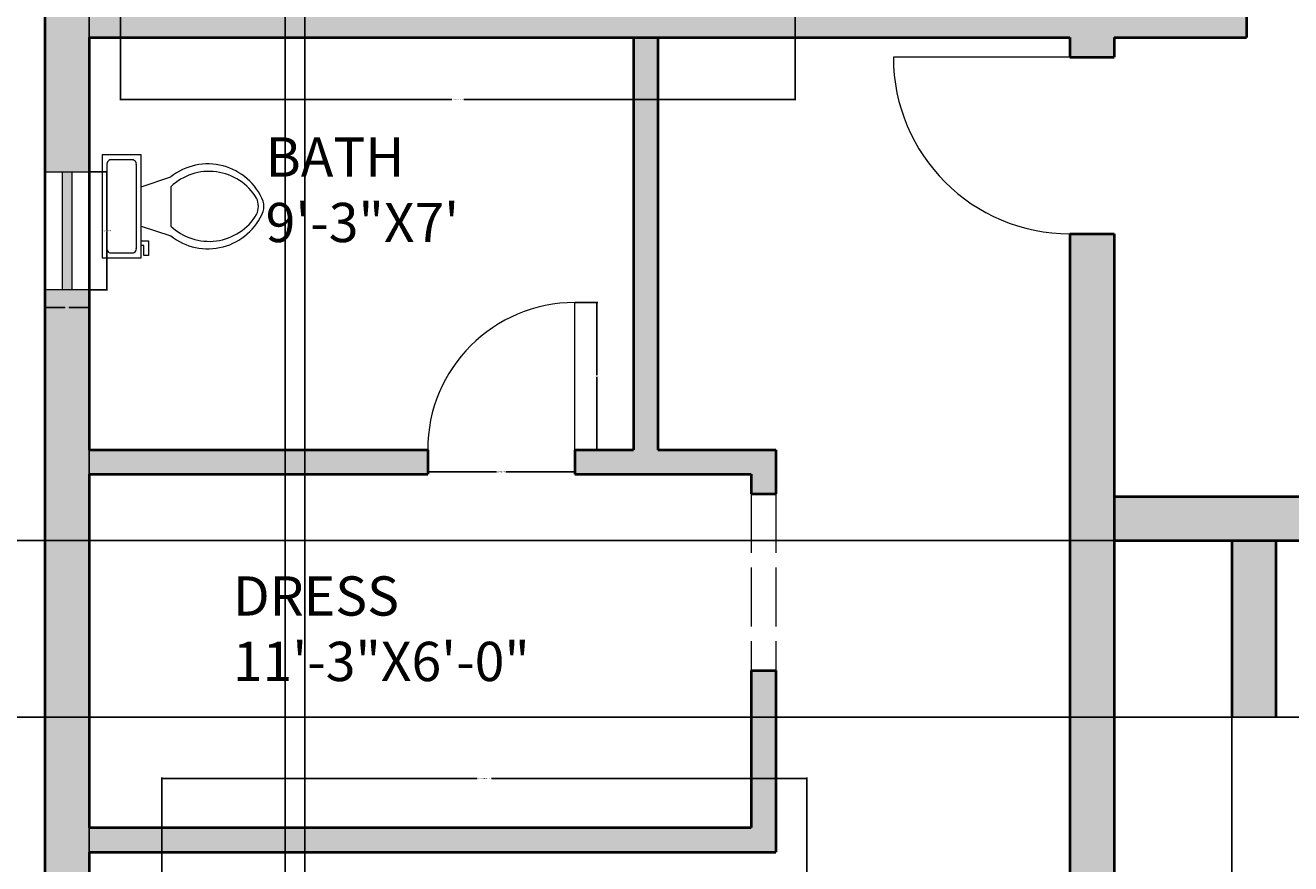
# Model space of a CAD drawing. Units: inches. Extents: x 2330 to 3943, y 1763 to 3461.
# Tile 9 of 40: x 2472 to 2730, y 2383 to 2554. Entities that reach past the tile are written whole.
import ezdxf

# ---------------------------------------------------------------- set-up
doc = ezdxf.new("R2010")
doc.units = ezdxf.units.IN
doc.linetypes.add('ACAD_ISO02W100', pattern=[15, 12, -3])
for name, color, linetype, lineweight in [('A-ANNO-DIMS', 2, 'Continuous', 18), ('A-AREA-IDEN', 7, 'Continuous', 18), ('A-DOOR', 4, 'Continuous', 18), ('A-FLOR', 7, 'Continuous', 25), ('A-FLOR-FIXT', 8, 'Continuous', 18), ('A-GLAZ', 4, 'Continuous', 18), ('A-WALL', 7, 'Continuous', 40), ('A-WALL-OVHD', 7, 'ACAD_ISO02W100', 18), ('A-WALL-PATT', 252, 'Continuous', 13)]:
    doc.layers.add(name, color=color, linetype=linetype, lineweight=lineweight)
doc.styles.get("Standard").update_dxf_attribs({"font": 'arial.ttf'})
doc.dimstyles.get("Standard").update_dxf_attribs({"dimtxt": 0.18, "dimasz": 0.18, "dimexe": 0.18, "dimexo": 0.0625, "dimgap": 0.09, "dimtad": 0, "dimtih": 1, "dimtoh": 1, "dimdec": 4, "dimzin": 0, "dimdsep": 46, "dimtxsty": 'Standard', "dimcen": 0.09, "dimadec": 0, "dimazin": 0, "dimtfac": 1, "dimtdec": 4, "dimtofl": 0, "dimtmove": 0, "dimatfit": 3, "dimfxl": 1, "dimtolj": 1, "dimtzin": 0, "dimarcsym": 0})

# ---------------------------------------------------------------- blocks, each defined once
blk = doc.blocks.new('*U9')
for p, q in [((9.5, -6), (9.5, -2)), ((-10, -8.5), (-8, -8.5)), ((-10, -9.5), (-10, -8.5)), ((-7, -9.5), (-10, -9.5)), ((-8, -8.5), (-8, -8)), ((-7, -8), (-7, -9.5)), ((-4, -8), (-6, -14)), ((4, -8), (6, -14)), ((4, -14), (-4, -14))]:
    blk.add_line(p, q)
blk.add_lwpolyline([(10.5, -8), (10.5, 0), (-10.5, 0), (-10.5, -8)], close=True)
for points in [[(-9.5, -2), (-9.5, -6)], [(8.5, -1), (-8.5, -1)], [(-8.5, -7), (8.5, -7)]]:
    blk.add_lwpolyline(points)
for centre, radius, start, end in [((-8.62, -1.88), 0.884, 81.8699, 188.1301), ((8.62, -1.88), 0.884, 351.8699, 98.1301), ((-8.62, -6.12), 0.884, 171.8699, 278.1301), ((8.62, -6.12), 0.884, 261.8699, 8.1301), ((3.52, -21.58), 12.17, 141.4691, 247.9714), ((4.2, -21.82), 11.33, 136.3677, 238.9468), ((-3.52, -21.58), 12.17, 292.0284, 38.5307), ((-4.2, -21.82), 11.33, 301.053, 43.6321), ((0, -27.88), 4, 245.7318, 294.2682), ((0, -29), 4, 254.8605, 285.1395)]:
    blk.add_arc(centre, radius, start, end)
blk = doc.blocks.new('DOOR-SINGLE-36IN')
blk.add_line((0, 0), (-36, 0))
blk.add_arc((0, 0), 36, 180, 270)
blk = doc.blocks.new('DOOR-SINGLE-30IN')
blk.add_line((0, 0), (0, 30))
blk.add_arc((0, 0), 30, 90, 180)
blk = doc.blocks.new('WINDOW-24IN')
h = blk.add_hatch(color=256)
h.dxf.hatch_style = 1
h.paths.add_polyline_path([(5.5, 24), (3.5, 24), (3.5, 0), (5.5, 0)])
for p, q in [((9, 24), (0, 24)), ((3.5, 24), (3.5, 0)), ((5.5, 24), (5.5, 0)), ((9, 0), (0, 0))]:
    blk.add_line(p, q)
blk = doc.blocks.new('*D31')
at = {"layer": 'A-ANNO-DIMS', "color": 0, "lineweight": -2, "transparency": 16777216}
for p, q in [((2553.7, 2467.09), (2553.7, 2462.47)), ((2583.7, 2467.09), (2583.7, 2462.47)), ((2553.88, 2462.65), (2567.77, 2462.65)), ((2583.52, 2462.65), (2569.64, 2462.65))]:
    blk.add_line(p, q, dxfattribs=at)
at = {"layer": 'A-ANNO-DIMS', "color": 0, "transparency": 16777216}
for points in [[(2553.88, 2462.68), (2553.88, 2462.62), (2553.7, 2462.65)], [(2583.52, 2462.68), (2583.52, 2462.62), (2583.7, 2462.65)]]:
    blk.add_solid(points, dxfattribs=at)
at = {"layer": 'Defpoints', "color": 0, "transparency": 16777216}
for p in [(2553.7, 2467.15), (2583.7, 2467.15), (2583.7, 2462.65)]:
    blk.add_point(p, dxfattribs=at)
at = {"layer": 'A-ANNO-DIMS', "color": 0, "transparency": 16777216, "insert": (2568.7, 2462.65), "char_height": 0.18, "attachment_point": 5}
blk.add_mtext('\\A1;DOOR 30 TYP.', dxfattribs=at)
blk = doc.blocks.new('*D32')
at = {"layer": 'A-ANNO-DIMS', "color": 0, "lineweight": -2, "transparency": 16777216}
for p, q in [((2583.77, 2497.15), (2588.38, 2497.15)), ((2588.2, 2496.97), (2588.2, 2482.33)), ((2588.2, 2467.33), (2588.2, 2481.97)), ((2583.77, 2467.15), (2588.38, 2467.15))]:
    blk.add_line(p, q, dxfattribs=at)
at = {"layer": 'A-ANNO-DIMS', "color": 0, "transparency": 16777216}
for points in [[(2588.17, 2496.97), (2588.23, 2496.97), (2588.2, 2497.15)], [(2588.17, 2467.33), (2588.23, 2467.33), (2588.2, 2467.15)]]:
    blk.add_solid(points, dxfattribs=at)
at = {"layer": 'Defpoints', "color": 0, "transparency": 16777216}
for p in [(2583.7, 2497.15), (2588.2, 2497.15), (2583.7, 2467.15)]:
    blk.add_point(p, dxfattribs=at)
at = {"layer": 'A-ANNO-DIMS', "color": 0, "transparency": 16777216, "insert": (2588.2, 2482.15), "char_height": 0.18, "attachment_point": 5}
blk.add_mtext('\\A1;30 TYP.', dxfattribs=at)
blk = doc.blocks.new('*D37')
at = {"layer": 'A-ANNO-DIMS', "color": 0, "lineweight": -2, "transparency": 16777216}
for p, q in [((2484.72, 2523.76), (2488.44, 2523.76)), ((2488.26, 2523.58), (2488.26, 2511.94)), ((2488.26, 2499.94), (2488.26, 2511.57)), ((2484.72, 2499.76), (2488.44, 2499.76))]:
    blk.add_line(p, q, dxfattribs=at)
at = {"layer": 'A-ANNO-DIMS', "color": 0, "transparency": 16777216}
for points in [[(2488.23, 2523.58), (2488.29, 2523.58), (2488.26, 2523.76)], [(2488.23, 2499.94), (2488.29, 2499.94), (2488.26, 2499.76)]]:
    blk.add_solid(points, dxfattribs=at)
at = {"layer": 'Defpoints', "color": 0, "transparency": 16777216}
for p in [(2484.66, 2523.76), (2488.26, 2523.76), (2484.66, 2499.76)]:
    blk.add_point(p, dxfattribs=at)
at = {"layer": 'A-ANNO-DIMS', "color": 0, "transparency": 16777216, "insert": (2488.26, 2511.76), "char_height": 0.18, "attachment_point": 5}
blk.add_mtext('\\A1;WINDOW 24 TYP.', dxfattribs=at)
blk = doc.blocks.new('*D38')
at = {"layer": 'A-ANNO-DIMS', "color": 0, "lineweight": -2, "transparency": 16777216}
for p, q in [((2475.66, 2499.69), (2475.66, 2495.98)), ((2484.66, 2499.69), (2484.66, 2495.98)), ((2475.84, 2496.16), (2479.7, 2496.16)), ((2484.48, 2496.16), (2480.62, 2496.16))]:
    blk.add_line(p, q, dxfattribs=at)
at = {"layer": 'A-ANNO-DIMS', "color": 0, "transparency": 16777216}
for points in [[(2475.84, 2496.19), (2475.84, 2496.13), (2475.66, 2496.16)], [(2484.48, 2496.19), (2484.48, 2496.13), (2484.66, 2496.16)]]:
    blk.add_solid(points, dxfattribs=at)
at = {"layer": 'Defpoints', "color": 0, "transparency": 16777216}
for p in [(2475.66, 2499.76), (2484.66, 2499.76), (2484.66, 2496.16)]:
    blk.add_point(p, dxfattribs=at)
at = {"layer": 'A-ANNO-DIMS', "color": 0, "transparency": 16777216, "insert": (2480.16, 2496.16), "char_height": 0.18, "attachment_point": 5}
blk.add_mtext('\\A1;9 TYP.', dxfattribs=at)
blk = doc.blocks.new('*D39')
at = {"layer": 'A-ANNO-DIMS', "color": 0, "lineweight": -2, "transparency": 16777216}
for p, q in [((2499.5, 2380.5), (2499.5, 2400.34)), ((2499.68, 2400.16), (2563.82, 2400.16)), ((2630.85, 2400.16), (2566.7, 2400.16)), ((2631.03, 2380.5), (2631.03, 2400.34))]:
    blk.add_line(p, q, dxfattribs=at)
at = {"layer": 'A-ANNO-DIMS', "color": 0, "transparency": 16777216}
for points in [[(2499.68, 2400.19), (2499.68, 2400.13), (2499.5, 2400.16)], [(2630.85, 2400.19), (2630.85, 2400.13), (2631.03, 2400.16)]]:
    blk.add_solid(points, dxfattribs=at)
at = {"layer": 'Defpoints', "color": 0, "transparency": 16777216}
for p in [(2631.03, 2400.16), (2499.5, 2380.43), (2631.03, 2380.43)]:
    blk.add_point(p, dxfattribs=at)
at = {"layer": 'A-ANNO-DIMS', "color": 0, "transparency": 16777216, "insert": (2565.26, 2400.16), "char_height": 0.18, "attachment_point": 5}
blk.add_mtext('\\A1;DOUBLE BED 132 TYP.', dxfattribs=at)
blk = doc.blocks.new('*D49')
at = {"layer": 'A-ANNO-DIMS', "color": 0, "lineweight": -2, "transparency": 16777216}
for p, q in [((2491.06, 2559.13), (2491.06, 2538.38)), ((2628.63, 2559.13), (2628.63, 2538.38)), ((2491.24, 2538.56), (2558.6, 2538.56)), ((2628.45, 2538.56), (2561.09, 2538.56))]:
    blk.add_line(p, q, dxfattribs=at)
at = {"layer": 'A-ANNO-DIMS', "color": 0, "transparency": 16777216}
for points in [[(2491.24, 2538.59), (2491.24, 2538.53), (2491.06, 2538.56)], [(2628.45, 2538.59), (2628.45, 2538.53), (2628.63, 2538.56)]]:
    blk.add_solid(points, dxfattribs=at)
at = {"layer": 'Defpoints', "color": 0, "transparency": 16777216}
for p in [(2491.06, 2559.19), (2628.63, 2559.19), (2491.06, 2538.56)]:
    blk.add_point(p, dxfattribs=at)
at = {"layer": 'A-ANNO-DIMS', "color": 0, "transparency": 16777216, "insert": (2559.84, 2538.56), "char_height": 0.18, "attachment_point": 5}
blk.add_mtext('\\A1;CORNER SOFA 138', dxfattribs=at)
blk = doc.blocks.new('*D62')
at = {"layer": 'A-ANNO-DIMS', "color": 0, "lineweight": -2, "transparency": 16777216}
for p, q in [((2475.6, 3162.65), (2330.5, 3162.65)), ((2330.68, 3162.47), (2330.68, 2687.58)), ((2330.68, 2212.33), (2330.68, 2687.22)), ((2475.6, 2212.15), (2330.5, 2212.15))]:
    blk.add_line(p, q, dxfattribs=at)
at = {"layer": 'A-ANNO-DIMS', "color": 0, "transparency": 16777216}
for points in [[(2330.65, 3162.47), (2330.71, 3162.47), (2330.68, 3162.65)], [(2330.65, 2212.33), (2330.71, 2212.33), (2330.68, 2212.15)]]:
    blk.add_solid(points, dxfattribs=at)
at = {"layer": 'Defpoints', "color": 0, "transparency": 16777216}
for p in [(2330.68, 3162.65), (2475.66, 3162.65), (2475.66, 2212.15)]:
    blk.add_point(p, dxfattribs=at)
at = {"layer": 'A-ANNO-DIMS', "color": 0, "transparency": 16777216, "insert": (2330.68, 2687.4), "char_height": 0.18, "attachment_point": 5}
blk.add_mtext('\\A1;950.5', dxfattribs=at)
blk = doc.blocks.new('*D77')
at = {"layer": 'A-ANNO-DIMS', "color": 0, "lineweight": -2, "transparency": 16777216}
for p, q in [((2717.66, 2412.59), (2717.66, 1901.2)), ((2944.66, 2412.59), (2944.66, 1901.2)), ((2717.84, 1901.38), (2830.87, 1901.38)), ((2944.48, 1901.38), (2831.45, 1901.38))]:
    blk.add_line(p, q, dxfattribs=at)
at = {"layer": 'A-ANNO-DIMS', "color": 0, "transparency": 16777216}
for points in [[(2717.84, 1901.41), (2717.84, 1901.35), (2717.66, 1901.38)], [(2944.48, 1901.41), (2944.48, 1901.35), (2944.66, 1901.38)]]:
    blk.add_solid(points, dxfattribs=at)
at = {"layer": 'Defpoints', "color": 0, "transparency": 16777216}
for p in [(2717.66, 2412.65), (2944.66, 2412.65), (2944.66, 1901.38)]:
    blk.add_point(p, dxfattribs=at)
at = {"layer": 'A-ANNO-DIMS', "color": 0, "transparency": 16777216, "insert": (2831.16, 1901.38), "char_height": 0.18, "attachment_point": 5}
blk.add_mtext('\\A1;227', dxfattribs=at)
blk = doc.blocks.new('*D78')
at = {"layer": 'A-ANNO-DIMS', "color": 0, "lineweight": -2, "transparency": 16777216}
for p, q in [((2717.6, 2448.65), (2330.5, 2448.65)), ((2330.68, 2448.47), (2330.68, 2430.83)), ((2330.68, 2412.83), (2330.68, 2430.47)), ((2717.6, 2412.65), (2330.5, 2412.65))]:
    blk.add_line(p, q, dxfattribs=at)
at = {"layer": 'A-ANNO-DIMS', "color": 0, "transparency": 16777216}
for points in [[(2330.65, 2448.47), (2330.71, 2448.47), (2330.68, 2448.65)], [(2330.65, 2412.83), (2330.71, 2412.83), (2330.68, 2412.65)]]:
    blk.add_solid(points, dxfattribs=at)
at = {"layer": 'Defpoints', "color": 0, "transparency": 16777216}
for p in [(2330.68, 2448.65), (2717.66, 2448.65), (2717.66, 2412.65)]:
    blk.add_point(p, dxfattribs=at)
at = {"layer": 'A-ANNO-DIMS', "color": 0, "transparency": 16777216, "insert": (2330.68, 2430.65), "char_height": 0.18, "attachment_point": 5}
blk.add_mtext('\\A1;36', dxfattribs=at)
blk = doc.blocks.new('*D79')
at = {"layer": 'A-ANNO-DIMS', "color": 0, "lineweight": -2, "transparency": 16777216}
for p, q in [((2484.66, 2221.21), (2484.66, 3461.3)), ((2484.84, 3461.12), (2504.44, 3461.12)), ((2524.48, 3461.12), (2504.88, 3461.12)), ((2524.66, 2221.21), (2524.66, 3461.3))]:
    blk.add_line(p, q, dxfattribs=at)
at = {"layer": 'A-ANNO-DIMS', "color": 0, "transparency": 16777216}
for points in [[(2484.84, 3461.15), (2484.84, 3461.09), (2484.66, 3461.12)], [(2524.48, 3461.15), (2524.48, 3461.09), (2524.66, 3461.12)]]:
    blk.add_solid(points, dxfattribs=at)
at = {"layer": 'Defpoints', "color": 0, "transparency": 16777216}
for p in [(2524.66, 3461.12), (2484.66, 2221.15), (2524.66, 2221.15)]:
    blk.add_point(p, dxfattribs=at)
at = {"layer": 'A-ANNO-DIMS', "color": 0, "transparency": 16777216, "insert": (2504.66, 3461.12), "char_height": 0.18, "attachment_point": 5}
blk.add_mtext('\\A1;40', dxfattribs=at)
blk = doc.blocks.new('*D90')
at = {"layer": 'A-ANNO-DIMS', "color": 0, "lineweight": -2, "transparency": 16777216}
for p, q in [((2484.66, 3153.59), (2484.66, 1901.2)), ((2528.66, 3153.59), (2528.66, 1901.2)), ((2484.84, 1901.38), (2506.44, 1901.38)), ((2528.48, 1901.38), (2506.88, 1901.38))]:
    blk.add_line(p, q, dxfattribs=at)
at = {"layer": 'A-ANNO-DIMS', "color": 0, "transparency": 16777216}
for points in [[(2484.84, 1901.41), (2484.84, 1901.35), (2484.66, 1901.38)], [(2528.48, 1901.41), (2528.48, 1901.35), (2528.66, 1901.38)]]:
    blk.add_solid(points, dxfattribs=at)
at = {"layer": 'Defpoints', "color": 0, "transparency": 16777216}
for p in [(2484.66, 3153.65), (2528.66, 3153.65), (2528.66, 1901.38)]:
    blk.add_point(p, dxfattribs=at)
at = {"layer": 'A-ANNO-DIMS', "color": 0, "transparency": 16777216, "insert": (2506.66, 1901.38), "char_height": 0.18, "attachment_point": 5}
blk.add_mtext('\\A1;44', dxfattribs=at)

msp = doc.modelspace()

# ---------------------------------------------------------------- hatches: boundary and pattern name
at = {"layer": 'A-WALL-PATT'}
h = msp.add_hatch(color=256, dxfattribs=at)
h.dxf.hatch_style = 1
h.paths.add_polyline_path([(2484.6605, 2594.4024), (2475.6605, 2594.4024), (2475.6605, 2523.7574), (2484.6605, 2523.7574), (2484.6605, 2551.1524), (2684.6605, 2551.1524), (2684.6605, 2547.1524), (2693.6605, 2547.1524), (2693.6605, 2551.1524), (2720.6605, 2551.1524), (2720.6605, 2560.1524), (2711.6605, 2560.1524), (2711.6605, 2556.1524), (2484.6605, 2556.1524)])
h = msp.add_hatch(color=256, dxfattribs=at)
h.dxf.hatch_style = 1
h.paths.add_polyline_path([(2600.6605, 2551.1524), (2595.6605, 2551.1524), (2595.6605, 2467.1524), (2583.7039, 2467.1524), (2583.7039, 2462.1524), (2619.6605, 2462.1524), (2619.6605, 2458.1524), (2624.6605, 2458.1524), (2624.6605, 2467.1524), (2600.6605, 2467.1524)])
h = msp.add_hatch(color=256, dxfattribs=at)
h.dxf.hatch_style = 1
h.paths.add_polyline_path([(2693.6605, 2511.1524), (2684.6605, 2511.1524), (2684.6605, 2221.1524), (2644.6605, 2221.1524), (2644.6605, 2212.1524), (2693.6605, 2212.1524)])
h = msp.add_hatch(color=256, dxfattribs=at)
h.dxf.hatch_style = 1
h.paths.add_polyline_path([(2484.6605, 2499.7574), (2475.6605, 2499.7574), (2475.6605, 2212.1524), (2524.6605, 2212.1524), (2524.6605, 2221.1524), (2484.6605, 2221.1524), (2484.6605, 2385.1524), (2624.6605, 2385.1524), (2624.6605, 2422.1524), (2619.6605, 2422.1524), (2619.6605, 2390.1524), (2484.6605, 2390.1524), (2484.6605, 2462.1524), (2553.7039, 2462.1524), (2553.7039, 2467.1524), (2484.6605, 2467.1524)])
h = msp.add_hatch(color=256, dxfattribs=at)
h.dxf.hatch_style = 1
h.paths.add_polyline_path([(2807.1605, 2457.6524), (2693.6605, 2457.6524), (2693.6605, 2448.6524), (2807.1605, 2448.6524)])
h = msp.add_hatch(color=256, dxfattribs=at)
h.dxf.hatch_style = 1
h.paths.add_polyline_path([(2726.6605, 2448.6524), (2717.6605, 2448.6524), (2717.6605, 2412.6524), (2726.6605, 2412.6524)])

# ---------------------------------------------------------------- linework, layer by layer
at = {"layer": 'A-FLOR'}
msp.add_line((2717.6605, 2412.6524), (2755.0816, 2412.6524), dxfattribs=at)
at = {"layer": 'A-WALL'}
for p, q in [((2475.6605, 3162.6524), (2475.6605, 2212.1524)), ((2720.6605, 2560.1524), (2720.6605, 2551.1524)), ((2484.6605, 2551.1524), (2684.6605, 2551.1524)), ((2484.6605, 2551.1524), (2484.6605, 2467.1524)), ((2595.6605, 2551.1524), (2595.6605, 2467.1524)), ((2600.6605, 2551.1524), (2600.6605, 2467.1524)), ((2684.6605, 2551.1524), (2684.6605, 2547.1524)), ((2693.6605, 2551.1524), (2693.6605, 2547.1524)), ((2693.6605, 2551.1524), (2720.6605, 2551.1524)), ((2684.6605, 2547.1524), (2693.6605, 2547.1524)), ((2684.6605, 2511.1524), (2693.6605, 2511.1524)), ((2684.6605, 2511.1524), (2684.6605, 2221.1524)), ((2693.6605, 2511.1524), (2693.6605, 2212.1524)), ((2484.6605, 2467.1524), (2553.7039, 2467.1524)), ((2553.7039, 2467.1524), (2553.7039, 2462.1524)), ((2583.7039, 2467.1524), (2583.7039, 2462.1524)), ((2583.7039, 2467.1524), (2595.6605, 2467.1524)), ((2600.6605, 2467.1524), (2624.6605, 2467.1524)), ((2624.6605, 2467.1524), (2624.6605, 2458.1524)), ((2484.6605, 2462.1524), (2553.7039, 2462.1524)), ((2484.6605, 2462.1524), (2484.6605, 2390.1524)), ((2583.7039, 2462.1524), (2619.6605, 2462.1524)), ((2619.6605, 2462.1524), (2619.6605, 2458.1524)), ((2619.6605, 2458.1524), (2624.6605, 2458.1524)), ((2693.6605, 2457.6524), (2807.1605, 2457.6524)), ((2693.6605, 2448.6524), (2807.1605, 2448.6524)), ((2717.6605, 2448.6524), (2717.6605, 2412.6524)), ((2726.6605, 2448.6524), (2726.6605, 2412.6524)), ((2619.6605, 2422.1524), (2624.6605, 2422.1524)), ((2619.6605, 2422.1524), (2619.6605, 2390.1524)), ((2624.6605, 2422.1524), (2624.6605, 2385.1524)), ((2484.6605, 2390.1524), (2619.6605, 2390.1524)), ((2484.6605, 2385.1524), (2624.6605, 2385.1524)), ((2484.6605, 2385.1524), (2484.6605, 2221.1524))]:
    msp.add_line(p, q, dxfattribs=at)
at = {"layer": 'A-WALL-OVHD'}
for p, q in [((2619.6605, 2458.1524), (2619.6605, 2422.1524)), ((2624.6605, 2458.1524), (2624.6605, 2422.1524))]:
    msp.add_line(p, q, dxfattribs=at)

# ---------------------------------------------------------------- block references
at = {"layer": 'A-DOOR'}
for name, p in [('DOOR-SINGLE-36IN', (2684.6605, 2547.1524)), ('DOOR-SINGLE-30IN', (2583.7039, 2467.1524))]:
    msp.add_blockref(name, p, dxfattribs=at)
at = {"layer": 'A-FLOR-FIXT', "rotation": 90}
msp.add_blockref('*U9', (2487.3074, 2516.7527), dxfattribs=at)
at = {"layer": 'A-GLAZ'}
msp.add_blockref('WINDOW-24IN', (2475.6605, 2499.7574), dxfattribs=at)

# ---------------------------------------------------------------- texts
at = {"layer": 'A-AREA-IDEN', "char_height": 8, "attachment_point": 1}
for s, width, insert in [('BATH\\P9\'-3"X7\'', 45.897347, (2520.6642, 2530.8065)), ('DRESS\\P11\'-3"X6\'-0"', 95.560425, (2513.989, 2441.3477))]:
    msp.add_mtext_dynamic_manual_height_columns(s, width=width, gutter_width=12.5, heights=[0], dxfattribs=dict(at, insert=insert))

# ---------------------------------------------------------------- dimensions: what is measured, and where the dimension line sits
at = {"layer": 'A-ANNO-DIMS'}
for base, p1, p2, picture, middle in [((2524.6605, 3461.1231), (2484.6605, 2221.1524), (2524.6605, 2221.1524), '*D79', (2504.6605, 3461.1231)), ((2528.6605, 1901.3774), (2484.6605, 3153.6524), (2528.6605, 3153.6524), '*D90', (2506.6605, 1901.3774)), ((2944.6605, 1901.3774), (2717.6605, 2412.6524), (2944.6605, 2412.6524), '*D77', (2831.1605, 1901.3774))]:
    dim = msp.add_linear_dim(base=base, p1=p1, p2=p2, dimstyle='Standard', override={"dimdec": 0, "dimlfac": 1, "dimrnd": 0, "dimzin": 0, "dimdsep": 46, "dimlunit": 2}, dxfattribs=at)
    dim.commit()
    dim.dimension.update_dxf_attribs({"geometry": picture, "text_midpoint": middle})
for base, p1, p2, override, picture, middle in [((2330.6824, 3162.6524), (2475.6605, 2212.1524), (2475.6605, 3162.6524), {"dimdec": 1, "dimlfac": 1, "dimrnd": 0, "dimzin": 0, "dimdsep": 46, "dimlunit": 2}, '*D62', (2330.6824, 2687.4024)), ((2330.6824, 2448.6524), (2717.6605, 2412.6524), (2717.6605, 2448.6524), {"dimdec": 0, "dimlfac": 1, "dimrnd": 0, "dimzin": 0, "dimdsep": 46, "dimlunit": 2}, '*D78', (2330.6824, 2430.6524))]:
    dim = msp.add_linear_dim(base=base, p1=p1, p2=p2, angle=90, dimstyle='Standard', override=override, dxfattribs=at)
    dim.commit()
    dim.dimension.update_dxf_attribs({"geometry": picture, "text_midpoint": middle})
for base, p1, p2, angle, text, picture, middle in [((2491.0616, 2538.5559), (2628.6266, 2559.1906), (2491.0616, 2559.1906), 180, 'CORNER SOFA <>', '*D49', (2559.8441, 2538.5559)), ((2488.2605, 2523.7574), (2484.6605, 2499.7574), (2484.6605, 2523.7574), 90, 'WINDOW <> TYP.', '*D37', (2488.2605, 2511.7574)), ((2588.2039, 2497.1524), (2583.7039, 2467.1524), (2583.7039, 2497.1524), 90, '<> TYP.', '*D32', (2588.2039, 2482.1524))]:
    dim = msp.add_linear_dim(base=base, p1=p1, p2=p2, angle=angle, text=text, dimstyle='Standard', override={"dimdec": 0, "dimlfac": 1, "dimrnd": 0, "dimzin": 0, "dimdsep": 46, "dimlunit": 2}, dxfattribs=at)
    dim.commit()
    dim.dimension.update_dxf_attribs({"geometry": picture, "text_midpoint": middle})
for base, p1, p2, text, picture, middle in [((2484.6605, 2496.1574), (2475.6605, 2499.7574), (2484.6605, 2499.7574), '<> TYP.', '*D38', (2480.1605, 2496.1574)), ((2583.7039, 2462.6524), (2553.7039, 2467.1524), (2583.7039, 2467.1524), 'DOOR <> TYP.', '*D31', (2568.7039, 2462.6524)), ((2631.0254, 2400.1629), (2499.4986, 2380.4339), (2631.0254, 2380.4339), 'DOUBLE BED <> TYP.', '*D39', (2565.262, 2400.1629))]:
    dim = msp.add_linear_dim(base=base, p1=p1, p2=p2, text=text, dimstyle='Standard', override={"dimdec": 0, "dimlfac": 1, "dimrnd": 0, "dimzin": 0, "dimdsep": 46, "dimlunit": 2}, dxfattribs=at)
    dim.commit()
    dim.dimension.update_dxf_attribs({"geometry": picture, "text_midpoint": middle})

doc.saveas('drawing.dxf')
